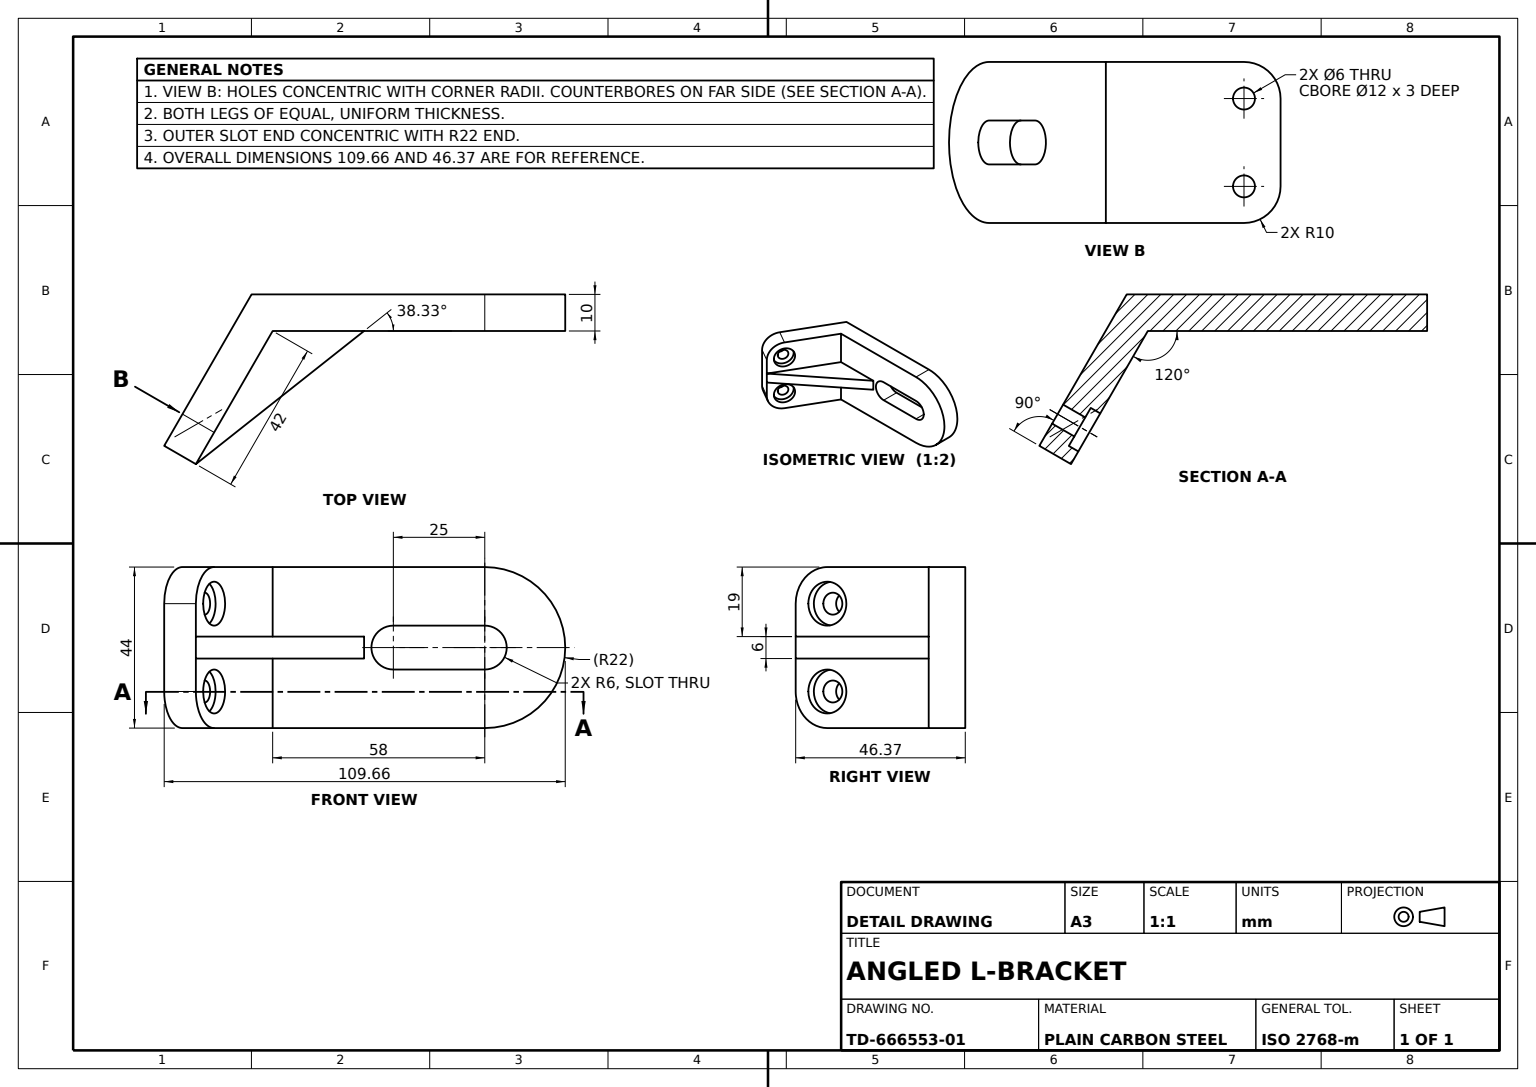
from build123d import *

# Parameters (mm, degrees)
BASE_PLATE_SKETCH_W        = 58
BASE_PLATE_SKETCH_H        = 44
BASE_PLATE_58X44X10_DEPTH  = 10
BASE_ROUNDED_END_SKETCH_R  = 22
BASE_ROUNDED_END_R22_DEPTH = 10
BASE_SLOT_DEPTH            = 10
ANGLED_ARM_120DEG_DEPTH    = 44
ARM_END_TRIM_DEPTH         = 10
COUNTERBORE_SKETCH_R       = 6
COUNTERBORES_2X_12X3_DEPTH = 3
ARM_HOLE_SKETCH_R          = 3
ARM_HOLES_2X_6_DEPTH       = 10
GUSSET_BLANK_DEPTH         = 44
GUSSET_SIDE_TRIM_1_DEPTH   = 19
GUSSET_SIDE_TRIM_2_DEPTH   = 19


with BuildPart() as part:
    # Base Plate Sketch → Base Plate 58x44x10 (new body)
    with BuildSketch(Plane.XY):
        with Locations((29, 22)):
            Rectangle(BASE_PLATE_SKETCH_W, BASE_PLATE_SKETCH_H)
    extrude(amount=BASE_PLATE_58X44X10_DEPTH)

    # Base Rounded End Sketch → Base Rounded End R22 (add)
    with BuildSketch(Plane.XY.offset(10)):
        with Locations((58, 22)):
            Circle(BASE_ROUNDED_END_SKETCH_R)
    extrude(amount=-BASE_ROUNDED_END_R22_DEPTH)

    # Base Slot Sketch → Base Slot (cut)
    with BuildSketch(Plane.XY.offset(10)):
        with BuildLine():
            Line((33, 28), (58, 28))
            ThreePointArc((58, 28), (64, 22), (58, 16))
            Line((58, 16), (33, 16))
            ThreePointArc((33, 16), (27, 22), (33, 28))
        make_face()
    extrude(amount=-BASE_SLOT_DEPTH, mode=Mode.SUBTRACT)

    # Angled Arm Sketch → Angled Arm 120deg (add)
    with BuildSketch(Plane.XZ):
        Polygon((-29.660254038, 41.373066959), (-5.773502692, 0), (0, 0), (0, 10), (-21, 46.373066959), align=None)
    extrude(amount=-ANGLED_ARM_120DEG_DEPTH)

    # Arm End Trim Sketch → Arm End Trim (cut)
    with BuildSketch(Plane(origin=(4.330127019, 0, 2.5), x_dir=(0.5000000000000042, 0, -0.8660254037844363), z_dir=(0.8660254037844363, 0, 0.5000000000000042))):
        with BuildLine():
            Line((-50.660254038, 0), (-40.660254038, 0))
            ThreePointArc((-40.660254038, 0), (-47.73132185, 2.928932188), (-50.660254038, 10))
            Line((-50.660254038, 10), (-50.660254038, 0))
        make_face()
        with BuildLine():
            Line((-50.660254038, 44), (-40.660254038, 44))
            ThreePointArc((-40.660254038, 44), (-47.73132185, 41.071067812), (-50.660254038, 34))
            Line((-50.660254038, 34), (-50.660254038, 44))
        make_face()
    extrude(amount=-ARM_END_TRIM_DEPTH, mode=Mode.SUBTRACT)

    # Counterbore Sketch → Counterbores 2xØ12x3 (cut)
    with BuildSketch(Plane(origin=(4.330127019, 0, 2.5), x_dir=(0.5000000000000042, 0, -0.8660254037844363), z_dir=(0.8660254037844363, 0, 0.5000000000000042))):
        with Locations((-40.660254038, 34)):
            Circle(COUNTERBORE_SKETCH_R)
        with Locations((-40.660254038, 10)):
            Circle(COUNTERBORE_SKETCH_R)
    extrude(amount=-COUNTERBORES_2X_12X3_DEPTH, mode=Mode.SUBTRACT)

    # Arm Hole Sketch → Arm Holes 2xØ6 (cut)
    with BuildSketch(Plane(origin=(1.732050808, 0, 1), x_dir=(0.5000000000000042, 0, -0.8660254037844363), z_dir=(0.8660254037844363, 0, 0.5000000000000042))):
        with Locations((-40.660254038, 34)):
            Circle(ARM_HOLE_SKETCH_R)
        with Locations((-40.660254038, 10)):
            Circle(ARM_HOLE_SKETCH_R)
    extrude(amount=-ARM_HOLES_2X_6_DEPTH, mode=Mode.SUBTRACT)

    # Gusset Profile Sketch → Gusset Blank (add)
    with BuildSketch(Plane.XZ):
        Polygon((0, 10), (25, 10), (-21, 46.373066959), align=None)
    extrude(amount=-GUSSET_BLANK_DEPTH)

    # Gusset Side Trim 1 Sketch → Gusset Side Trim 1 (cut)
    with BuildSketch(Plane.XZ):
        Polygon((4.891585761, 10), (25, 10), (-21, 46.373066959), (0, 10), align=None)
    extrude(amount=-GUSSET_SIDE_TRIM_1_DEPTH, mode=Mode.SUBTRACT)

    # Gusset Side Trim 2 Sketch → Gusset Side Trim 2 (cut)
    with BuildSketch(Plane(origin=(0, 44, 0), x_dir=(1, 0, 0), z_dir=(0, 1, 0))):
        Polygon((25, -10), (0, -10), (-21, -46.373066959), align=None)
    extrude(amount=-GUSSET_SIDE_TRIM_2_DEPTH, mode=Mode.SUBTRACT)


solid = part.part
